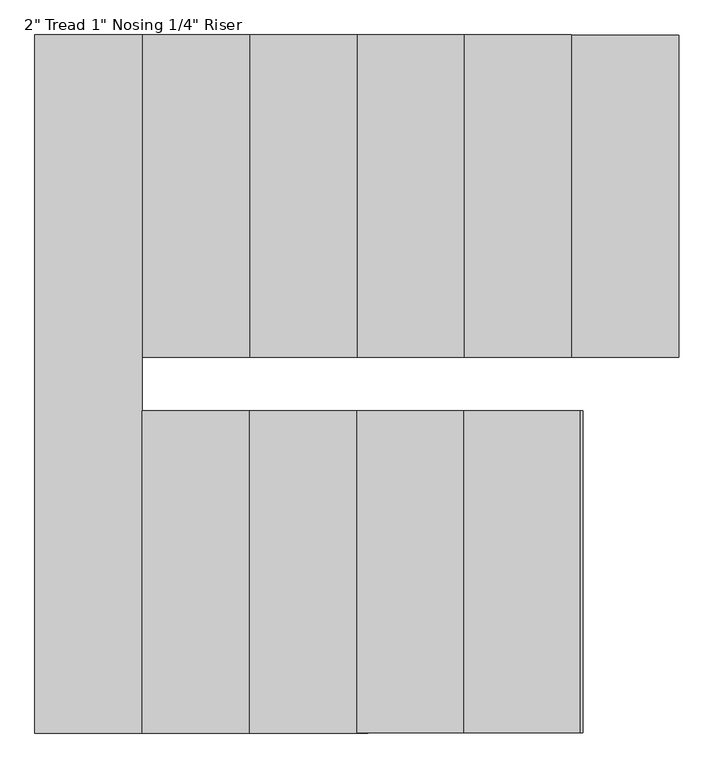
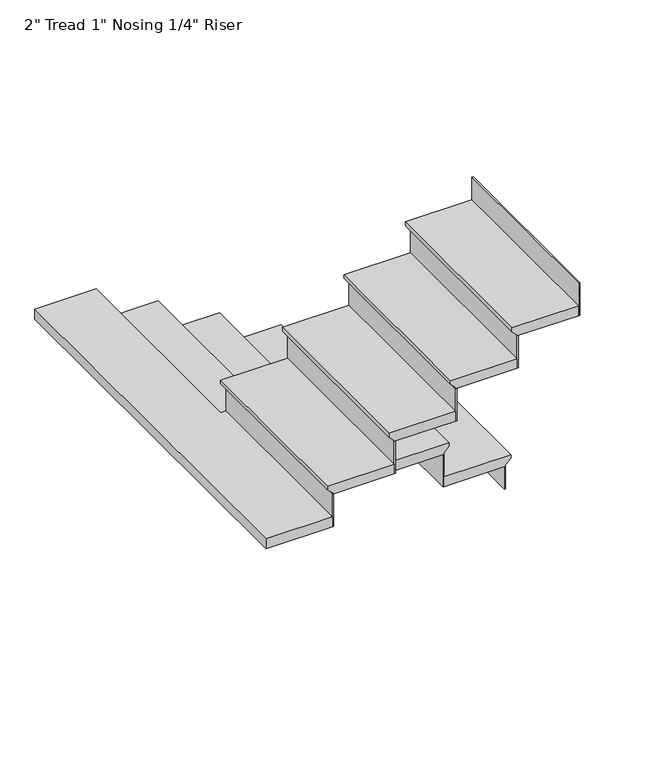
"""IFC4 building model written with IfcOpenShell, lengths in millimetres: stair flight geometry."""

from ifc_helpers import new_model, si_unit, origin, place, context, project, spatial, faceted_brep, source, transform, mapped, element, save


def stair_flight_b60de328(model_context):
    return source(origin(), model_context, "Body", "Brep", [
        faceted_brep([(3327.4, 3340.1, 3198.2833333), (3327.4, 3340.1, 3217.3333333), (3327.4, 2425.7, 3217.3333333), (3327.4, 2425.7, 3198.2833333), (3302.0, 3340.1, 3172.8833333), (3302.0, 2425.7, 3172.8833333), (2997.2, 3340.1, 3217.3333333), (2997.2, 2425.7, 3217.3333333), (3302.0, 2425.7, 3166.5333333), (2997.2, 2425.7, 3166.5333333), (2997.2, 3340.1, 3166.5333333), (3302.0, 3340.1, 3166.5333333)], [[[0, 1, 2, 3]], [[4, 0, 3, 5]], [[2, 1, 6, 7]], [[8, 9, 10, 11]], [[2, 7, 9, 8, 5, 3]], [[8, 11, 4, 5]], [[6, 1, 0, 4, 11, 10]], [[7, 6, 10, 9]]]),
        faceted_brep([(3302.0, 3340.1, 3166.5333333), (3302.0, 3340.1, 3048.0), (3295.65, 3340.1, 3048.0), (3295.65, 3340.1, 3166.5333333), (3302.0, 2425.7, 3166.5333333), (3295.65, 2425.7, 3166.5333333), (3295.65, 2425.7, 3048.0), (3302.0, 2425.7, 3048.0)], [[[0, 1, 2, 3]], [[4, 5, 6, 7]], [[1, 0, 4, 7]], [[2, 1, 7, 6]], [[3, 2, 6, 5]], [[0, 3, 5, 4]]]),
        faceted_brep([(2997.2, 3340.1, 3335.8666667), (2997.2, 3340.1, 3166.5333333), (2990.85, 3340.1, 3166.5333333), (2990.85, 3340.1, 3335.8666667), (2997.2, 2425.7, 3335.8666667), (2990.85, 2425.7, 3335.8666667), (2990.85, 2425.7, 3166.5333333), (2997.2, 2425.7, 3166.5333333)], [[[0, 1, 2, 3]], [[4, 5, 6, 7]], [[1, 0, 4, 7]], [[2, 1, 7, 6]], [[3, 2, 6, 5]], [[0, 3, 5, 4]]]),
        faceted_brep([(3022.6, 2425.7, 3386.6666667), (3022.6, 3340.1, 3386.6666667), (2692.4, 3340.1, 3386.6666667), (2692.4, 2425.7, 3386.6666667), (2997.2, 2425.7, 3335.8666667), (2692.4, 2425.7, 3335.8666667), (2692.4, 3340.1, 3335.8666667), (2997.2, 3340.1, 3335.8666667), (2997.2, 2425.7, 3342.2166667), (3022.6, 2425.7, 3367.6166667), (2997.2, 3340.1, 3342.2166667), (3022.6, 3340.1, 3367.6166667)], [[[0, 1, 2, 3]], [[4, 5, 6, 7]], [[0, 3, 5, 4, 8, 9]], [[4, 7, 10, 8]], [[2, 1, 11, 10, 7, 6]], [[3, 2, 6, 5]], [[11, 1, 0, 9]], [[10, 11, 9, 8]]]),
        faceted_brep([(2692.4, 3340.1, 3505.2), (2692.4, 3340.1, 3335.8666667), (2686.05, 3340.1, 3335.8666667), (2686.05, 3340.1, 3505.2), (2692.4, 2425.7, 3505.2), (2686.05, 2425.7, 3505.2), (2686.05, 2425.7, 3335.8666667), (2692.4, 2425.7, 3335.8666667)], [[[0, 1, 2, 3]], [[4, 5, 6, 7]], [[1, 0, 4, 7]], [[2, 1, 7, 6]], [[3, 2, 6, 5]], [[0, 3, 5, 4]]]),
        faceted_brep([(2717.8, 2425.7, 3556.0), (2717.8, 3340.1, 3556.0), (2387.6, 3340.1, 3556.0), (2387.6, 2425.7, 3556.0), (2692.4, 2425.7, 3505.2), (2387.6, 2425.7, 3505.2), (2387.6, 3340.1, 3505.2), (2692.4, 3340.1, 3505.2), (2692.4, 2425.7, 3511.55), (2717.8, 2425.7, 3536.95), (2692.4, 3340.1, 3511.55), (2717.8, 3340.1, 3536.95)], [[[0, 1, 2, 3]], [[4, 5, 6, 7]], [[0, 3, 5, 4, 8, 9]], [[4, 7, 10, 8]], [[2, 1, 11, 10, 7, 6]], [[3, 2, 6, 5]], [[11, 1, 0, 9]], [[10, 11, 9, 8]]]),
        faceted_brep([(2387.6, 3340.1, 3674.5333333), (2387.6, 3340.1, 3505.2), (2381.25, 3340.1, 3505.2), (2381.25, 3340.1, 3674.5333333), (2387.6, 2425.7, 3674.5333333), (2381.25, 2425.7, 3674.5333333), (2381.25, 2425.7, 3505.2), (2387.6, 2425.7, 3505.2)], [[[0, 1, 2, 3]], [[4, 5, 6, 7]], [[1, 0, 4, 7]], [[2, 1, 7, 6]], [[3, 2, 6, 5]], [[0, 3, 5, 4]]]),
        faceted_brep([(2413.0, 2425.7, 3725.3333333), (2413.0, 3340.1, 3725.3333333), (2082.8, 3340.1, 3725.3333333), (2082.8, 2425.7, 3725.3333333), (2387.6, 2425.7, 3674.5333333), (2082.8, 2425.7, 3674.5333333), (2082.8, 3340.1, 3674.5333333), (2387.6, 3340.1, 3674.5333333), (2387.6, 2425.7, 3680.8833333), (2413.0, 2425.7, 3706.2833333), (2387.6, 3340.1, 3680.8833333), (2413.0, 3340.1, 3706.2833333)], [[[0, 1, 2, 3]], [[4, 5, 6, 7]], [[0, 3, 5, 4, 8, 9]], [[4, 7, 10, 8]], [[2, 1, 11, 10, 7, 6]], [[3, 2, 6, 5]], [[11, 1, 0, 9]], [[10, 11, 9, 8]]]),
        faceted_brep([(2082.8, 3340.1, 3843.8666667), (2082.8, 3340.1, 3674.5333333), (2076.45, 3340.1, 3674.5333333), (2076.45, 3340.1, 3843.8666667), (2082.8, 2425.7, 3843.8666667), (2076.45, 2425.7, 3843.8666667), (2076.45, 2425.7, 3674.5333333), (2082.8, 2425.7, 3674.5333333)], [[[0, 1, 2, 3]], [[4, 5, 6, 7]], [[1, 0, 4, 7]], [[2, 1, 7, 6]], [[3, 2, 6, 5]], [[0, 3, 5, 4]]]),
        faceted_brep([(2108.2, 2425.7, 3894.6666667), (2108.2, 3340.1, 3894.6666667), (1778.0, 3340.1, 3894.6666667), (1778.0, 2425.7, 3894.6666667), (2082.8, 2425.7, 3843.8666667), (1778.0, 2425.7, 3843.8666667), (1778.0, 3340.1, 3843.8666667), (2082.8, 3340.1, 3843.8666667), (2082.8, 2425.7, 3850.2166667), (2108.2, 2425.7, 3875.6166667), (2082.8, 3340.1, 3850.2166667), (2108.2, 3340.1, 3875.6166667)], [[[0, 1, 2, 3]], [[4, 5, 6, 7]], [[0, 3, 5, 4, 8, 9]], [[4, 7, 10, 8]], [[2, 1, 11, 10, 7, 6]], [[3, 2, 6, 5]], [[11, 1, 0, 9]], [[10, 11, 9, 8]]]),
        faceted_brep([(1778.0, 3340.1, 4013.2), (1778.0, 3340.1, 3843.8666667), (1771.65, 3340.1, 3843.8666667), (1771.65, 3340.1, 4013.2), (1778.0, 2425.7, 4013.2), (1771.65, 2425.7, 4013.2), (1771.65, 2425.7, 3843.8666667), (1778.0, 2425.7, 3843.8666667)], [[[0, 1, 2, 3]], [[4, 5, 6, 7]], [[1, 0, 4, 7]], [[2, 1, 7, 6]], [[3, 2, 6, 5]], [[0, 3, 5, 4]]]),
        faceted_brep([(1828.8, 2273.3, 4064.0), (1803.4, 2273.3, 4064.0), (1803.4, 3340.1, 4064.0), (1498.6, 3340.1, 4064.0), (1498.6, 1358.9, 4064.0), (1828.8, 1358.9, 4064.0), (1803.4, 2273.3, 4013.2), (1828.8, 2273.3, 4013.2), (1828.8, 1358.9, 4013.2), (1498.6, 1358.9, 4013.2), (1498.6, 3340.1, 4013.2), (1778.0, 3340.1, 4013.2), (1778.0, 2425.7, 4013.2), (1803.4, 2425.7, 4013.2), (1803.4, 2425.7, 4044.95), (1803.4, 3340.1, 4044.95), (1778.0, 2425.7, 4019.55), (1778.0, 3340.1, 4019.55)], [[[0, 1, 2, 3, 4, 5]], [[6, 7, 8, 9, 10, 11, 12, 13]], [[1, 0, 7, 6]], [[2, 1, 6, 13, 14, 15]], [[13, 12, 16, 14]], [[12, 11, 17, 16]], [[3, 2, 15, 17, 11, 10]], [[4, 3, 10, 9]], [[5, 4, 9, 8]], [[0, 5, 8, 7]], [[17, 15, 14, 16]]]),
        faceted_brep([(1828.8, 1358.9, 4182.5333333), (1828.8, 1358.9, 4013.2), (1835.15, 1358.9, 4013.2), (1835.15, 1358.9, 4182.5333333), (1828.8, 2273.3, 4182.5333333), (1835.15, 2273.3, 4182.5333333), (1835.15, 2273.3, 4013.2), (1828.8, 2273.3, 4013.2)], [[[0, 1, 2, 3]], [[4, 5, 6, 7]], [[1, 0, 4, 7]], [[2, 1, 7, 6]], [[3, 2, 6, 5]], [[0, 3, 5, 4]]]),
        faceted_brep([(1803.4, 2273.3, 4233.3333333), (1803.4, 1358.9, 4233.3333333), (2133.6, 1358.9, 4233.3333333), (2133.6, 2273.3, 4233.3333333), (1828.8, 2273.3, 4182.5333333), (2133.6, 2273.3, 4182.5333333), (2133.6, 1358.9, 4182.5333333), (1828.8, 1358.9, 4182.5333333), (1828.8, 2273.3, 4188.8833333), (1803.4, 2273.3, 4214.2833333), (1828.8, 1358.9, 4188.8833333), (1803.4, 1358.9, 4214.2833333)], [[[0, 1, 2, 3]], [[4, 5, 6, 7]], [[0, 3, 5, 4, 8, 9]], [[4, 7, 10, 8]], [[2, 1, 11, 10, 7, 6]], [[3, 2, 6, 5]], [[11, 1, 0, 9]], [[10, 11, 9, 8]]]),
        faceted_brep([(2133.6, 1358.9, 4351.8666667), (2133.6, 1358.9, 4182.5333333), (2139.95, 1358.9, 4182.5333333), (2139.95, 1358.9, 4351.8666667), (2133.6, 2273.3, 4351.8666667), (2139.95, 2273.3, 4351.8666667), (2139.95, 2273.3, 4182.5333333), (2133.6, 2273.3, 4182.5333333)], [[[0, 1, 2, 3]], [[4, 5, 6, 7]], [[1, 0, 4, 7]], [[2, 1, 7, 6]], [[3, 2, 6, 5]], [[0, 3, 5, 4]]]),
        faceted_brep([(2108.2, 2273.3, 4402.6666667), (2108.2, 1358.9, 4402.6666667), (2438.4, 1358.9, 4402.6666667), (2438.4, 2273.3, 4402.6666667), (2133.6, 2273.3, 4351.8666667), (2438.4, 2273.3, 4351.8666667), (2438.4, 1358.9, 4351.8666667), (2133.6, 1358.9, 4351.8666667), (2133.6, 2273.3, 4358.2166667), (2108.2, 2273.3, 4383.6166667), (2133.6, 1358.9, 4358.2166667), (2108.2, 1358.9, 4383.6166667)], [[[0, 1, 2, 3]], [[4, 5, 6, 7]], [[0, 3, 5, 4, 8, 9]], [[4, 7, 10, 8]], [[2, 1, 11, 10, 7, 6]], [[3, 2, 6, 5]], [[11, 1, 0, 9]], [[10, 11, 9, 8]]]),
        faceted_brep([(2438.4, 1358.9, 4521.2), (2438.4, 1358.9, 4351.8666667), (2444.75, 1358.9, 4351.8666667), (2444.75, 1358.9, 4521.2), (2438.4, 2273.3, 4521.2), (2444.75, 2273.3, 4521.2), (2444.75, 2273.3, 4351.8666667), (2438.4, 2273.3, 4351.8666667)], [[[0, 1, 2, 3]], [[4, 5, 6, 7]], [[1, 0, 4, 7]], [[2, 1, 7, 6]], [[3, 2, 6, 5]], [[0, 3, 5, 4]]]),
        faceted_brep([(2413.0, 2273.3, 4572.0), (2413.0, 1358.9, 4572.0), (2743.2, 1358.9, 4572.0), (2743.2, 2273.3, 4572.0), (2438.4, 2273.3, 4521.2), (2743.2, 2273.3, 4521.2), (2743.2, 1358.9, 4521.2), (2438.4, 1358.9, 4521.2), (2438.4, 2273.3, 4527.55), (2413.0, 2273.3, 4552.95), (2438.4, 1358.9, 4527.55), (2413.0, 1358.9, 4552.95)], [[[0, 1, 2, 3]], [[4, 5, 6, 7]], [[0, 3, 5, 4, 8, 9]], [[4, 7, 10, 8]], [[2, 1, 11, 10, 7, 6]], [[3, 2, 6, 5]], [[11, 1, 0, 9]], [[10, 11, 9, 8]]]),
        faceted_brep([(2743.2, 1358.9, 4690.5333333), (2743.2, 1358.9, 4521.2), (2749.55, 1358.9, 4521.2), (2749.55, 1358.9, 4690.5333333), (2743.2, 2273.3, 4690.5333333), (2749.55, 2273.3, 4690.5333333), (2749.55, 2273.3, 4521.2), (2743.2, 2273.3, 4521.2)], [[[0, 1, 2, 3]], [[4, 5, 6, 7]], [[1, 0, 4, 7]], [[2, 1, 7, 6]], [[3, 2, 6, 5]], [[0, 3, 5, 4]]]),
        faceted_brep([(3048.0, 1358.9, 4859.8666667), (3048.0, 1358.9, 4690.5333333), (3054.35, 1358.9, 4690.5333333), (3054.35, 1358.9, 4859.8666667), (3048.0, 2273.3, 4859.8666667), (3054.35, 2273.3, 4859.8666667), (3054.35, 2273.3, 4690.5333333), (3048.0, 2273.3, 4690.5333333)], [[[0, 1, 2, 3]], [[4, 5, 6, 7]], [[1, 0, 4, 7]], [[2, 1, 7, 6]], [[3, 2, 6, 5]], [[0, 3, 5, 4]]]),
        faceted_brep([(2717.8, 2273.3, 4741.3333333), (2717.8, 1358.9, 4741.3333333), (3048.0, 1358.9, 4741.3333333), (3048.0, 2273.3, 4741.3333333), (2743.2, 2273.3, 4690.5333333), (3048.0, 2273.3, 4690.5333333), (3048.0, 1358.9, 4690.5333333), (2743.2, 1358.9, 4690.5333333), (2743.2, 2273.3, 4696.8833333), (2717.8, 2273.3, 4722.2833333), (2743.2, 1358.9, 4696.8833333), (2717.8, 1358.9, 4722.2833333)], [[[0, 1, 2, 3]], [[4, 5, 6, 7]], [[0, 3, 5, 4, 8, 9]], [[4, 7, 10, 8]], [[2, 1, 11, 10, 7, 6]], [[3, 2, 6, 5]], [[11, 1, 0, 9]], [[10, 11, 9, 8]]]),
    ])


if __name__ == "__main__":
    model = new_model("IFC4")
    model_context = context("Model", 3, world=origin())
    ifc_project = project(units=[si_unit("LENGTHUNIT", "METRE", prefix="MILLI")], contexts=[model_context])
    site = spatial("IfcSite", under=ifc_project)
    building = spatial("IfcBuilding", under=site)
    placement = place(None, origin())
    stair_flight_shape = stair_flight_b60de328(model_context)
    element("IfcStairFlight", 1, ObjectType="2\" Tread 1\" Nosing 1/4\" Riser", at=placement, inside=building, context=model_context, shape_type="MappedRepresentation", body=[
        mapped(stair_flight_shape, transform((0.0, 0.0, 0.0), x_axis=(1.0, 0.0, 0.0), y_axis=(0.0, 1.0, 0.0), z_axis=(0.0, 0.0, 1.0))),
    ])
    save(model, "model.ifc")
